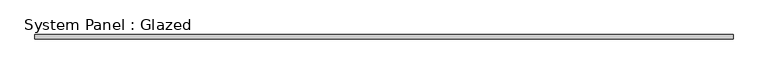
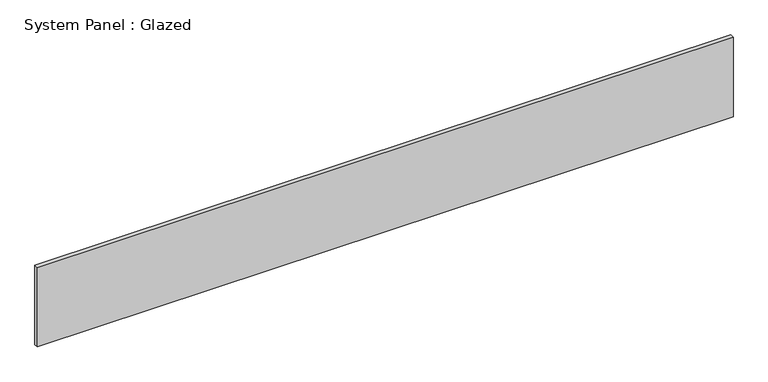
"""IFC4 building model written with IfcOpenShell, lengths in millimetres: plate geometry, System Panel : Glazed."""

from ifc_helpers import new_model, si_unit, origin, origin_with_axes, place, context, project, spatial, polyline, outline, extrude, source, transform, mapped, element, save


def system_panel_glazed_289ab79d(model_context):
    return source(origin(), model_context, "Body", "SweptSolid", [
        extrude(outline(polyline([(2057.4, -44.45), (-2057.4, -44.45), (-2057.4, -19.05), (2057.4, -19.05), (2057.4, -44.45)])), origin_with_axes(), (0.0, 0.0, 1.0), 495.3),
    ])


if __name__ == "__main__":
    model = new_model("IFC4")
    model_context = context("Model", 3, world=origin())
    ifc_project = project(units=[si_unit("LENGTHUNIT", "METRE", prefix="MILLI")], contexts=[model_context])
    site = spatial("IfcSite", under=ifc_project)
    building = spatial("IfcBuilding", under=site)
    placement = place(None, origin())
    system_panel_glazed_shape = system_panel_glazed_289ab79d(model_context)
    element("IfcPlate", 1, ObjectType="System Panel : Glazed", at=placement, inside=building, context=model_context, shape_type="MappedRepresentation", body=[
        mapped(system_panel_glazed_shape, transform((0.0, 0.0, 0.0), x_axis=(1.0, 0.0, 0.0), y_axis=(0.0, 1.0, 0.0), z_axis=(0.0, 0.0, 1.0))),
    ])
    save(model, "model.ifc")

# Revit data of these elements
# Type "System Panel : Glazed"
#   Construction Type Id = "GSP4R"
#   Analytic Construction = "1/8 in Pilkington single glazing"
#   Visual Light Transmittance = 0.9
#   Solar Heat Gain Coefficient = 0.86
#   Heat Transfer Coefficient (U) = 1.18115 BTU/(h·ft²·°F)
#   Define Thermal Properties by = 1
# Element 1 (IfcPlate, "System Panel : Glazed")
#   Materials on its faces: "Glass"
# Materials
#   "Glass": class "Glass", colour RGB 0 128 192, transparency 0.75, Description = "Soda Lime Glass", Cost = 0
